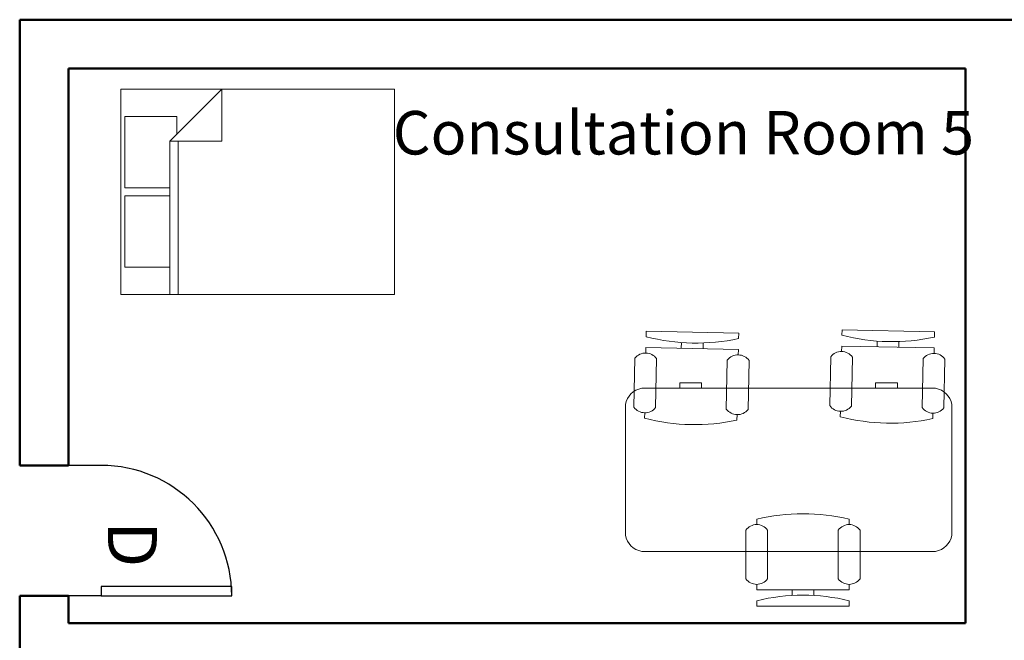
# Model space of a CAD drawing. Units: inches. Extents: x -364 to 705, y -52 to 1250.
# Tile 27 of 34: x 185 to 366, y 648 to 762. Entities that reach past the tile are written whole.
import ezdxf

# ---------------------------------------------------------------- set-up
doc = ezdxf.new("R2010")
doc.units = ezdxf.units.IN
doc.header["$MEASUREMENT"] = 0
for name, color, linetype, lineweight in [('A-ANNO-IDEN', 1, 'Continuous', 18), ('A-AREA-IDEN', 3, 'Continuous', 18), ('A-DOOR', 1, 'Continuous', 25), ('A-FURN', 8, 'Continuous', 18), ('A-WALL', 41, 'Continuous', 50)]:
    doc.layers.add(name, color=color, linetype=linetype, lineweight=lineweight)
doc.styles.get("Standard").update_dxf_attribs({"font": 'arial.ttf'})

# ---------------------------------------------------------------- blocks, each defined once
blk = doc.blocks.new('Chair - Desk')
for p, q in [((-8.5, 0), (-8.5, -1)), ((-8.5, 0), (8.5, 0)), ((8.5, 0), (8.5, -1)), ((-8.5, -3), (-8.5, -4)), ((-8.5, -3), (8.5, -3)), ((-2, -3), (-2, -1.9355)), ((2, -1.9576), (2, -3)), ((8.5, -3), (8.5, -4)), ((-10.5, -5), (-10.5, -14)), ((-6.5, -14), (-6.5, -5)), ((6.5, -5), (6.5, -14)), ((10.5, -14), (10.5, -5)), ((-8.5, -15), (-8.5, -16)), ((8.5, -15), (8.5, -16))]:
    blk.add_line(p, q)
for centre, radius, start, end in [((0, 34.625), 36.625, 256.5803, 283.4197), ((-8.5, -6.5), 2.5, 36.8699, 143.1301), ((8.5, -6.5), 2.5, 36.8699, 143.1301), ((-8.5, -12.5), 2.5, 216.8699, 323.1301), ((8.5, -12.5), 2.5, 216.8699, 323.1301), ((0, 19.625), 36.625, 256.5803, 283.4197)]:
    blk.add_arc(centre, radius, start, end)
blk = doc.blocks.new('Desk - 30 x 60 in.')
for p, q in [((-26.999995, 0), (26.999995, 0)), ((-29.999995, -27), (-29.999995, -3)), ((29.999995, -3), (29.999995, -27)), ((26.999995, -30), (-26.999995, -30)), ((-20.000005, -30), (-20.000005, -31)), ((-16.000005, -31), (-16.000005, -30)), ((15.999995, -31), (15.999995, -30)), ((19.999995, -30), (19.999995, -31)), ((-20.000005, -31), (-16.000005, -31)), ((19.999995, -31), (15.999995, -31))]:
    blk.add_line(p, q)
for centre, start, end in [((-26.499995, -3.5), 98.1301, 171.8699), ((26.499995, -3.5), 8.130102, 81.8699), ((-26.499995, -26.5), 188.1301, 261.8699), ((26.499995, -26.5), 278.1301, 351.8699)]:
    blk.add_arc(centre, 3.535534, start, end)
blk = doc.blocks.new('Bed - Queen')
for p, q in [((0, -80.00003), (0, 0)), ((0, 0), (59.99999, 0)), ((59.99999, 0), (59.99999, -80.00003)), ((7.99999, -1.2), (28.79998, -1.2)), ((7.99999, -14.4), (7.99999, -1.2)), ((28.79998, -1.2), (28.79998, -14.4)), ((31.19999, -1.2), (51.99999, -1.2)), ((31.19999, -14.4), (31.19999, -1.2)), ((51.99999, -1.2), (51.99999, -16.4)), ((0, -14.4), (44.8, -14.4)), ((44.8, -16.8), (0, -16.8)), ((59.99999, -29.6), (44.8, -14.4)), ((44.8, -14.4), (44.8, -29.6)), ((51.99999, -16.4), (46.79936, -16.4)), ((44.8, -29.6), (59.99999, -29.6)), ((59.99999, -80.00003), (0, -80.00003))]:
    blk.add_line(p, q)
blk = doc.blocks.new('*U14')
for p, q in [((0, 0), (0, -6)), ((-24, 0), (-24, -6))]:
    blk.add_line(p, q)
blk.add_lwpolyline([(0, 0), (0, 24), (-1.75, 24), (-1.75, 0)], close=True)
blk.add_arc((0, 0), 24, 90, 180)

msp = doc.modelspace()

# ---------------------------------------------------------------- linework, layer by layer
at = {"layer": 'A-WALL'}
for p, q in [((379.58, 762.11), (184.58, 762.11)), ((184.58, 680.11), (184.58, 762.11)), ((358.58, 753.11), (193.58, 753.11)), ((193.58, 680.11), (193.58, 753.11)), ((358.58, 651.11), (358.58, 753.11)), ((193.58, 680.11), (184.58, 680.11)), ((193.58, 656.11), (184.58, 656.11)), ((184.58, 551.11), (184.58, 656.11)), ((193.58, 651.11), (193.58, 656.11)), ((358.58, 651.11), (193.58, 651.11))]:
    msp.add_line(p, q, dxfattribs=at)

# ---------------------------------------------------------------- block references
at = {"layer": 'A-DOOR', "rotation": 270}
msp.add_blockref('*U14', (199.58, 656.11), dxfattribs=at)
at = {"layer": 'A-FURN', "xscale": 0.6293684586277993, "yscale": 0.6293684586277993, "zscale": 0.6293684586277993, "rotation": 90}
msp.add_blockref('Bed - Queen', (203.16, 711.56), dxfattribs=at)
at = {"layer": 'A-FURN'}
for name, p, rotation in [('Chair - Desk', (308.34, 704.62), 358.8399543093714), ('Chair - Desk', (344.35, 704.89), 358.8399543093714), ('Desk - 30 x 60 in.', (326.02, 664.3), 180), ('Chair - Desk', (328.65, 654.23), 180)]:
    msp.add_blockref(name, p, dxfattribs=dict(at, rotation=rotation))

# ---------------------------------------------------------------- texts
at = {"layer": 'A-ANNO-IDEN', "insert": (209.82, 669.82), "char_height": 9, "attachment_point": 1, "rotation": 270}
msp.add_mtext_dynamic_manual_height_columns('D', width=16.916, gutter_width=1, heights=[0], dxfattribs=at)
at = {"layer": 'A-AREA-IDEN', "insert": (253.2, 745.32), "char_height": 8, "attachment_point": 1}
msp.add_mtext_dynamic_manual_height_columns('Consultation Room 5', width=124.8937, gutter_width=1, heights=[0], dxfattribs=at)

doc.saveas('drawing.dxf')
